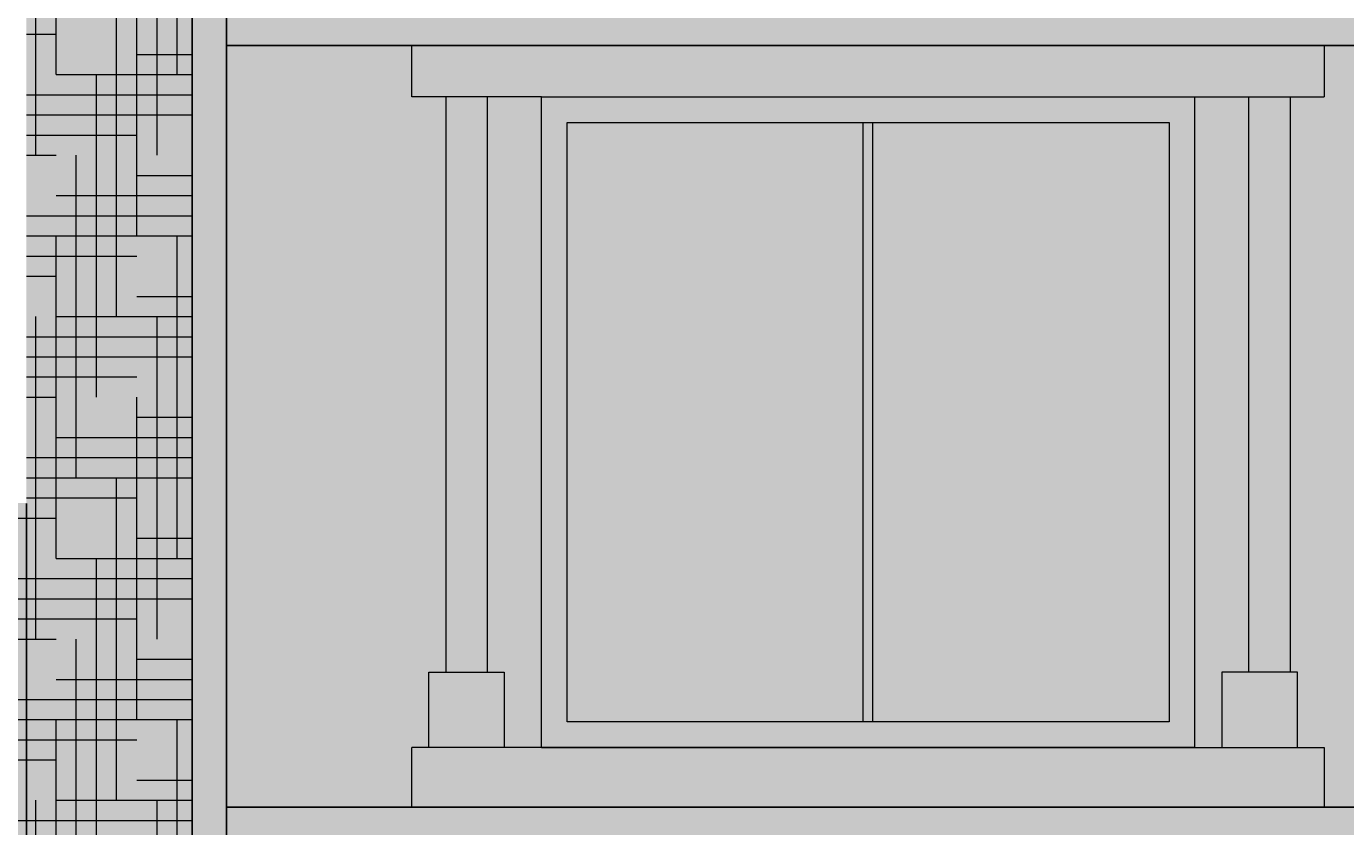
# Model space of a CAD drawing. Units: inches. Extents: x 3024 to 4744, y 1110 to 2100.
# Tile 15 of 29: x 3450 to 3657, y 1279 to 1405. Entities that reach past the tile are written whole.
import ezdxf

# ---------------------------------------------------------------- set-up
doc = ezdxf.new("R2010")
doc.units = ezdxf.units.IN
for name, color, linetype, lineweight in [('A-ANNO-DIMS', 2, 'Continuous', 18), ('A-ELEV', 7, 'Continuous', 25), ('A-ELEV-PATT', 252, 'Continuous', 13), ('A-GLAZ', 4, 'Continuous', 18)]:
    doc.layers.add(name, color=color, linetype=linetype, lineweight=lineweight)
doc.styles.get("Standard").update_dxf_attribs({"font": 'arial.ttf'})
doc.dimstyles.get("Standard").update_dxf_attribs({"dimtxt": 0.18, "dimasz": 0.18, "dimexe": 0.18, "dimexo": 0.0625, "dimgap": 0.09, "dimtad": 0, "dimtih": 1, "dimtoh": 1, "dimdec": 1, "dimzin": 0, "dimdsep": 46, "dimlunit": 3, "dimtxsty": 'Standard', "dimcen": 0.09, "dimadec": 0, "dimazin": 0, "dimtfac": 1, "dimtdec": 1, "dimtofl": 0, "dimtmove": 0, "dimatfit": 3, "dimfxl": 1, "dimtolj": 1, "dimtzin": 0, "dimarcsym": 0})

# ---------------------------------------------------------------- blocks, each defined once
blk = doc.blocks.new('WIN-BALCONY-A')
for p, q in [((3169.4, 1897.49), (3148.97, 1897.49)), ((3169.4, 1897.49), (3148.97, 1897.49)), ((3169.4, 1897.49), (3292.61, 1897.49)), ((3169.4, 1897.49), (3292.61, 1897.49)), ((3169.4, 1795.04), (3148.97, 1795.04)), ((3169.4, 1795.04), (3148.97, 1795.04)), ((3169.4, 1795.04), (3292.61, 1795.04)), ((3169.4, 1795.04), (3292.61, 1795.04))]:
    blk.add_line(p, q)
for points in [[(3148.97, 1897.49), (3148.97, 1905.61), (3292.61, 1905.61), (3292.61, 1897.49)], [(3148.97, 1897.49), (3148.97, 1905.61), (3292.61, 1905.61), (3292.61, 1897.49)], [(3292.61, 1795.04), (3292.61, 1785.61), (3148.97, 1785.61), (3148.97, 1795.04)], [(3292.61, 1795.04), (3292.61, 1785.61), (3148.97, 1785.61), (3148.97, 1795.04)]]:
    blk.add_lwpolyline(points)
for points in [[(3154.33, 1806.87), (3160.86, 1806.87), (3160.86, 1897.49), (3154.33, 1897.49)], [(3154.33, 1806.87), (3160.86, 1806.87), (3160.86, 1897.49), (3154.33, 1897.49)], [(3272.18, 1795.04), (3169.4, 1795.04), (3169.4, 1897.49), (3272.18, 1897.49)], [(3272.18, 1795.04), (3169.4, 1795.04), (3169.4, 1897.49), (3272.18, 1897.49)], [(3287.25, 1806.87), (3280.72, 1806.87), (3280.72, 1897.49), (3287.25, 1897.49)], [(3287.25, 1806.87), (3280.72, 1806.87), (3280.72, 1897.49), (3287.25, 1897.49)], [(3268.18, 1799.04), (3173.4, 1799.04), (3173.4, 1893.49), (3268.18, 1893.49)], [(3268.18, 1799.04), (3173.4, 1799.04), (3173.4, 1893.49), (3268.18, 1893.49)], [(3220.05, 1893.49), (3221.52, 1893.49), (3221.52, 1799.04), (3220.05, 1799.04)], [(3220.05, 1893.49), (3221.52, 1893.49), (3221.52, 1799.04), (3220.05, 1799.04)], [(3163.53, 1795.04), (3151.66, 1795.04), (3151.66, 1806.87), (3163.53, 1806.87)], [(3163.53, 1795.04), (3151.66, 1795.04), (3151.66, 1806.87), (3163.53, 1806.87)], [(3276.51, 1795.04), (3288.38, 1795.04), (3288.38, 1806.87), (3276.51, 1806.87)], [(3276.51, 1795.04), (3288.38, 1795.04), (3288.38, 1806.87), (3276.51, 1806.87)]]:
    blk.add_lwpolyline(points, close=True)
blk = doc.blocks.new('*D57')
at = {"layer": 'A-ANNO-DIMS', "color": 0, "lineweight": -2, "transparency": 16777216}
for p, q in [((3361.22, 1329.46), (3361.22, 1109.93)), ((3449.72, 1329.46), (3449.72, 1109.93)), ((3361.4, 1110.11), (3405.15, 1110.11)), ((3449.54, 1110.11), (3405.8, 1110.11))]:
    blk.add_line(p, q, dxfattribs=at)
at = {"layer": 'A-ANNO-DIMS', "color": 0, "transparency": 16777216}
for points in [[(3361.4, 1110.14), (3361.4, 1110.08), (3361.22, 1110.11)], [(3449.54, 1110.14), (3449.54, 1110.08), (3449.72, 1110.11)]]:
    blk.add_solid(points, dxfattribs=at)
at = {"layer": 'Defpoints', "color": 0, "transparency": 16777216}
for p in [(3361.22, 1329.52), (3449.72, 1329.52), (3449.72, 1110.11)]:
    blk.add_point(p, dxfattribs=at)
at = {"layer": 'A-ANNO-DIMS', "color": 0, "transparency": 16777216, "insert": (3405.47, 1110.11), "char_height": 0.18, "attachment_point": 5}
blk.add_mtext('\\A1;88.5', dxfattribs=at)
blk = doc.blocks.new('*D58')
at = {"layer": 'A-ANNO-DIMS', "color": 0, "lineweight": -2, "transparency": 16777216}
for p, q in [((3449.72, 1329.46), (3449.72, 1109.93)), ((3481.24, 1155.55), (3481.24, 1109.93)), ((3449.9, 1110.11), (3465.09, 1110.11)), ((3481.06, 1110.11), (3465.87, 1110.11))]:
    blk.add_line(p, q, dxfattribs=at)
at = {"layer": 'A-ANNO-DIMS', "color": 0, "transparency": 16777216}
for points in [[(3449.9, 1110.14), (3449.9, 1110.08), (3449.72, 1110.11)], [(3481.06, 1110.14), (3481.06, 1110.08), (3481.24, 1110.11)]]:
    blk.add_solid(points, dxfattribs=at)
at = {"layer": 'Defpoints', "color": 0, "transparency": 16777216}
for p in [(3449.72, 1329.52), (3481.24, 1155.61), (3481.24, 1110.11)]:
    blk.add_point(p, dxfattribs=at)
at = {"layer": 'A-ANNO-DIMS', "color": 0, "transparency": 16777216, "insert": (3465.48, 1110.11), "char_height": 0.18, "attachment_point": 5}
blk.add_mtext('\\A1;31.52', dxfattribs=at)
blk = doc.blocks.new('*D64')
at = {"layer": 'A-ANNO-DIMS', "color": 0, "lineweight": -2, "transparency": 16777216}
for p, q in [((3069.79, 1241.5), (3069.79, 2100.44)), ((3069.97, 2100.26), (3405.08, 2100.26)), ((3740.97, 2100.26), (3405.87, 2100.26)), ((3741.15, 1241.5), (3741.15, 2100.44))]:
    blk.add_line(p, q, dxfattribs=at)
at = {"layer": 'A-ANNO-DIMS', "color": 0, "transparency": 16777216}
for points in [[(3069.97, 2100.29), (3069.97, 2100.23), (3069.79, 2100.26)], [(3740.97, 2100.29), (3740.97, 2100.23), (3741.15, 2100.26)]]:
    blk.add_solid(points, dxfattribs=at)
at = {"layer": 'Defpoints', "color": 0, "transparency": 16777216}
for p in [(3741.15, 2100.26), (3069.79, 1241.43), (3741.15, 1241.43)]:
    blk.add_point(p, dxfattribs=at)
at = {"layer": 'A-ANNO-DIMS', "color": 0, "transparency": 16777216, "insert": (3405.47, 2100.26), "char_height": 0.18, "attachment_point": 5}
blk.add_mtext('\\A1;671.4', dxfattribs=at)
blk = doc.blocks.new('*D75')
at = {"layer": 'A-ANNO-DIMS', "color": 0, "lineweight": -2, "transparency": 16777216}
for p, q in [((3491.89, 2054.76), (3786.83, 2054.76)), ((3786.65, 2054.58), (3786.65, 1605.37)), ((3786.65, 1155.79), (3786.65, 1605)), ((3741.21, 1155.61), (3786.83, 1155.61))]:
    blk.add_line(p, q, dxfattribs=at)
at = {"layer": 'A-ANNO-DIMS', "color": 0, "transparency": 16777216}
for points in [[(3786.62, 2054.58), (3786.68, 2054.58), (3786.65, 2054.76)], [(3786.62, 1155.79), (3786.68, 1155.79), (3786.65, 1155.61)]]:
    blk.add_solid(points, dxfattribs=at)
at = {"layer": 'Defpoints', "color": 0, "transparency": 16777216}
for p in [(3491.83, 2054.76), (3786.65, 2054.76), (3741.15, 1155.61)]:
    blk.add_point(p, dxfattribs=at)
at = {"layer": 'A-ANNO-DIMS', "color": 0, "transparency": 16777216, "insert": (3786.65, 1605.18), "char_height": 0.18, "attachment_point": 5}
blk.add_mtext('\\A1;899.1', dxfattribs=at)

msp = doc.modelspace()

# ---------------------------------------------------------------- hatches: boundary and pattern name
at = {"layer": 'A-ELEV-PATT'}
h = msp.add_hatch(color=256, dxfattribs=at)
h.dxf.hatch_style = 1
h.paths.add_polyline_path([(3491.8271, 2054.7584), (3320.5658, 2054.7584), (3320.5658, 2043.5286), (3491.8271, 2043.5286)])
h.paths.add_polyline_path([(3292.6051, 1905.6112), (3148.9694, 1905.6112), (3148.9694, 1897.4879), (3169.3964, 1897.4879), (3292.6051, 1897.4879)])
h.paths.add_polyline_path([(3292.6051, 1795.0431), (3169.3964, 1795.0431), (3148.9694, 1795.0431), (3148.9694, 1785.6112), (3292.6051, 1785.6112)])
h.paths.add_polyline_path([(3292.6051, 1779.6112), (3148.9694, 1779.6112), (3148.9694, 1771.4879), (3169.3964, 1771.4879), (3292.6051, 1771.4879)])
h.paths.add_polyline_path([(3292.6051, 1669.0431), (3169.3964, 1669.0431), (3148.9694, 1669.0431), (3148.9694, 1659.6112), (3292.6051, 1659.6112)])
h.paths.add_polyline_path([(3292.6051, 1653.6112), (3148.9694, 1653.6112), (3148.9694, 1645.4879), (3169.3964, 1645.4879), (3292.6051, 1645.4879)])
h.paths.add_polyline_path([(3292.6051, 1543.0431), (3169.3964, 1543.0431), (3148.9694, 1543.0431), (3148.9694, 1533.6112), (3292.6051, 1533.6112)])
h.paths.add_polyline_path([(3292.6051, 1527.6112), (3148.9694, 1527.6112), (3148.9694, 1519.4879), (3169.3964, 1519.4879), (3292.6051, 1519.4879)])
h.paths.add_polyline_path([(3292.6051, 1401.6112), (3148.9694, 1401.6112), (3148.9694, 1393.4879), (3169.3964, 1393.4879), (3292.6051, 1393.4879)])
h.paths.add_polyline_path([(3292.6051, 1417.0431), (3169.3964, 1417.0431), (3148.9694, 1417.0431), (3148.9694, 1407.6112), (3292.6051, 1407.6112)])
h.paths.add_polyline_path([(3292.6051, 1291.0431), (3169.3964, 1291.0431), (3148.9694, 1291.0431), (3148.9694, 1281.6112), (3292.6051, 1281.6112)])
h.paths.add_polyline_path([(3654.037, 1165.0431), (3530.8283, 1165.0431), (3510.4013, 1165.0431), (3510.4013, 1155.6112), (3654.037, 1155.6112)])
h.paths.add_polyline_path([(3654.037, 1275.6112), (3510.4013, 1275.6112), (3510.4013, 1267.4879), (3530.8283, 1267.4879), (3654.037, 1267.4879)])
h.paths.add_polyline_path([(3654.037, 1291.0431), (3530.8283, 1291.0431), (3510.4013, 1291.0431), (3510.4013, 1281.6112), (3654.037, 1281.6112)])
h.paths.add_polyline_path([(3654.037, 1417.0431), (3530.8283, 1417.0431), (3510.4013, 1417.0431), (3510.4013, 1407.6112), (3654.037, 1407.6112)])
h.paths.add_polyline_path([(3654.037, 1401.6112), (3510.4013, 1401.6112), (3510.4013, 1393.4879), (3530.8283, 1393.4879), (3654.037, 1393.4879)])
h.paths.add_polyline_path([(3654.037, 1543.0431), (3530.8283, 1543.0431), (3510.4013, 1543.0431), (3510.4013, 1533.6112), (3654.037, 1533.6112)])
h.paths.add_polyline_path([(3654.037, 1527.6112), (3510.4013, 1527.6112), (3510.4013, 1519.4879), (3530.8283, 1519.4879), (3654.037, 1519.4879)])
h.paths.add_polyline_path([(3654.037, 1653.6112), (3510.4013, 1653.6112), (3510.4013, 1645.4879), (3530.8283, 1645.4879), (3654.037, 1645.4879)])
h.paths.add_polyline_path([(3654.037, 1669.0431), (3530.8283, 1669.0431), (3510.4013, 1669.0431), (3510.4013, 1659.6112), (3654.037, 1659.6112)])
h.paths.add_polyline_path([(3654.037, 1779.6112), (3510.4013, 1779.6112), (3510.4013, 1771.4879), (3530.8283, 1771.4879), (3654.037, 1771.4879)])
h.paths.add_polyline_path([(3654.037, 1795.0431), (3530.8283, 1795.0431), (3510.4013, 1795.0431), (3510.4013, 1785.6112), (3654.037, 1785.6112)])
h.paths.add_polyline_path([(3654.037, 1905.6112), (3510.4013, 1905.6112), (3510.4013, 1897.4879), (3530.8283, 1897.4879), (3654.037, 1897.4879)])
h = msp.add_hatch(color=256, dxfattribs=at)
h.dxf.hatch_style = 1
h.paths.add_polyline_path([(3335.1044, 2043.5286), (3329.7033, 2043.5286), (3329.7033, 1155.6112), (3335.1044, 1155.6112)])
h.paths.add_polyline_path([(3481.2411, 2043.5286), (3335.1044, 2043.5286), (3335.1044, 1155.6112), (3481.2411, 1155.6112)])
h.paths.add_polyline_path([(3449.7202, 1329.5246), (3361.2242, 1329.5246), (3361.2242, 1436.6064), (3449.7202, 1436.6064)], flags=16)
h.paths.add_polyline_path([(3445.7202, 1333.5246), (3365.2242, 1333.5246), (3365.2242, 1432.6064), (3445.7202, 1432.6064)], flags=0)
h.paths.add_polyline_path([(3449.7202, 1455.5246), (3361.2242, 1455.5246), (3361.2242, 1562.6064), (3449.7202, 1562.6064)], flags=16)
h.paths.add_polyline_path([(3445.7202, 1459.5246), (3365.2242, 1459.5246), (3365.2242, 1558.6064), (3445.7202, 1558.6064)], flags=0)
h.paths.add_polyline_path([(3449.7202, 1581.5246), (3361.2242, 1581.5246), (3361.2242, 1688.6064), (3449.7202, 1688.6064)], flags=16)
h.paths.add_polyline_path([(3445.7202, 1585.5246), (3365.2242, 1585.5246), (3365.2242, 1684.6064), (3445.7202, 1684.6064)], flags=0)
h.paths.add_polyline_path([(3449.7202, 1707.5246), (3361.2242, 1707.5246), (3361.2242, 1814.6064), (3449.7202, 1814.6064)], flags=16)
h.paths.add_polyline_path([(3445.7202, 1711.5246), (3365.2242, 1711.5246), (3365.2242, 1810.6064), (3445.7202, 1810.6064)], flags=0)
h.paths.add_polyline_path([(3449.7202, 1833.5246), (3361.2242, 1833.5246), (3361.2242, 1940.6064), (3449.7202, 1940.6064)], flags=16)
h.paths.add_polyline_path([(3445.7202, 1837.5246), (3365.2242, 1837.5246), (3365.2242, 1936.6064), (3445.7202, 1936.6064)], flags=0)
h = msp.add_hatch(color=256, dxfattribs=at)
h.dxf.hatch_style = 1
h.paths.add_polyline_path([(3475.84, 2043.5286), (3335.1044, 2043.5286), (3335.1044, 1155.6112), (3475.84, 1155.6112)])
h.paths.add_polyline_path([(3449.7202, 1940.6064), (3449.7202, 1833.5246), (3361.2242, 1833.5246), (3361.2242, 1940.6064)], flags=16)
h.paths.add_polyline_path([(3445.7202, 1936.6064), (3445.7202, 1837.5246), (3365.2242, 1837.5246), (3365.2242, 1936.6064)], flags=0)
h.paths.add_polyline_path([(3449.7202, 1814.6064), (3449.7202, 1707.5246), (3361.2242, 1707.5246), (3361.2242, 1814.6064)], flags=16)
h.paths.add_polyline_path([(3445.7202, 1810.6064), (3445.7202, 1711.5246), (3365.2242, 1711.5246), (3365.2242, 1810.6064)], flags=0)
h.paths.add_polyline_path([(3449.7202, 1688.6064), (3449.7202, 1581.5246), (3361.2242, 1581.5246), (3361.2242, 1688.6064)], flags=16)
h.paths.add_polyline_path([(3445.7202, 1684.6064), (3445.7202, 1585.5246), (3365.2242, 1585.5246), (3365.2242, 1684.6064)], flags=0)
h.paths.add_polyline_path([(3449.7202, 1562.6064), (3449.7202, 1455.5246), (3361.2242, 1455.5246), (3361.2242, 1562.6064)], flags=16)
h.paths.add_polyline_path([(3445.7202, 1558.6064), (3445.7202, 1459.5246), (3365.2242, 1459.5246), (3365.2242, 1558.6064)], flags=0)
h.paths.add_polyline_path([(3449.7202, 1436.6064), (3449.7202, 1329.5246), (3361.2242, 1329.5246), (3361.2242, 1436.6064)], flags=16)
h.paths.add_polyline_path([(3445.7202, 1432.6064), (3445.7202, 1333.5246), (3365.2242, 1333.5246), (3365.2242, 1432.6064)], flags=0)
h = msp.add_hatch(dxfattribs=at)
h.set_pattern_fill('HOUND', color=256, scale=2)
h.paths.add_polyline_path([(3475.84, 2043.5286), (3335.1044, 2043.5286), (3335.1044, 1155.6112), (3475.84, 1155.6112)])
h.paths.add_polyline_path([(3449.7202, 1940.6064), (3449.7202, 1833.5246), (3361.2242, 1833.5246), (3361.2242, 1940.6064)], flags=16)
h.paths.add_polyline_path([(3445.7202, 1936.6064), (3445.7202, 1837.5246), (3365.2242, 1837.5246), (3365.2242, 1936.6064)], flags=0)
h.paths.add_polyline_path([(3449.7202, 1814.6064), (3449.7202, 1707.5246), (3361.2242, 1707.5246), (3361.2242, 1814.6064)], flags=16)
h.paths.add_polyline_path([(3445.7202, 1810.6064), (3445.7202, 1711.5246), (3365.2242, 1711.5246), (3365.2242, 1810.6064)], flags=0)
h.paths.add_polyline_path([(3449.7202, 1688.6064), (3449.7202, 1581.5246), (3361.2242, 1581.5246), (3361.2242, 1688.6064)], flags=16)
h.paths.add_polyline_path([(3445.7202, 1684.6064), (3445.7202, 1585.5246), (3365.2242, 1585.5246), (3365.2242, 1684.6064)], flags=0)
h.paths.add_polyline_path([(3449.7202, 1562.6064), (3449.7202, 1455.5246), (3361.2242, 1455.5246), (3361.2242, 1562.6064)], flags=16)
h.paths.add_polyline_path([(3445.7202, 1558.6064), (3445.7202, 1459.5246), (3365.2242, 1459.5246), (3365.2242, 1558.6064)], flags=0)
h.paths.add_polyline_path([(3449.7202, 1436.6064), (3449.7202, 1329.5246), (3361.2242, 1329.5246), (3361.2242, 1436.6064)], flags=16)
h.paths.add_polyline_path([(3445.7202, 1432.6064), (3445.7202, 1333.5246), (3365.2242, 1333.5246), (3365.2242, 1432.6064)], flags=0)
h = msp.add_hatch(color=256, dxfattribs=at)
h.dxf.hatch_style = 1
h.paths.add_polyline_path([(3154.3287, 1897.4879), (3148.9694, 1897.4879), (3148.9694, 1905.6112), (3105.4722, 1905.6112), (3105.4722, 1785.6112), (3148.9694, 1785.6112), (3148.9694, 1795.0431), (3151.6604, 1795.0431), (3151.6604, 1806.8674), (3154.3287, 1806.8674)])
h.paths.add_polyline_path([(3329.7033, 1905.6112), (3292.6051, 1905.6112), (3292.6051, 1897.4879), (3287.2458, 1897.4879), (3287.2458, 1806.8674), (3288.3759, 1806.8674), (3288.3759, 1795.0431), (3292.6051, 1795.0431), (3292.6051, 1785.6112), (3329.7033, 1785.6112)])
h.paths.add_polyline_path([(3154.3287, 1771.4879), (3148.9694, 1771.4879), (3148.9694, 1779.6112), (3105.4722, 1779.6112), (3105.4722, 1659.6112), (3148.9694, 1659.6112), (3148.9694, 1669.0431), (3151.6604, 1669.0431), (3151.6604, 1680.8674), (3154.3287, 1680.8674)])
h.paths.add_polyline_path([(3329.7033, 1779.6112), (3292.6051, 1779.6112), (3292.6051, 1771.4879), (3287.2458, 1771.4879), (3287.2458, 1680.8674), (3288.3759, 1680.8674), (3288.3759, 1669.0431), (3292.6051, 1669.0431), (3292.6051, 1659.6112), (3329.7033, 1659.6112)])
h.paths.add_polyline_path([(3154.3287, 1645.4879), (3148.9694, 1645.4879), (3148.9694, 1653.6112), (3105.4722, 1653.6112), (3105.4722, 1533.6112), (3148.9694, 1533.6112), (3148.9694, 1543.0431), (3151.6604, 1543.0431), (3151.6604, 1554.8674), (3154.3287, 1554.8674)])
h.paths.add_polyline_path([(3329.7033, 1653.6112), (3292.6051, 1653.6112), (3292.6051, 1645.4879), (3287.2458, 1645.4879), (3287.2458, 1554.8674), (3288.3759, 1554.8674), (3288.3759, 1543.0431), (3292.6051, 1543.0431), (3292.6051, 1533.6112), (3329.7033, 1533.6112)])
h.paths.add_polyline_path([(3329.7033, 1527.6112), (3292.6051, 1527.6112), (3292.6051, 1519.4879), (3287.2458, 1519.4879), (3287.2458, 1428.8674), (3288.3759, 1428.8674), (3288.3759, 1417.0431), (3292.6051, 1417.0431), (3292.6051, 1407.6112), (3329.7033, 1407.6112)])
h.paths.add_polyline_path([(3329.7033, 1401.6112), (3292.6051, 1401.6112), (3292.6051, 1393.4879), (3287.2458, 1393.4879), (3287.2458, 1302.8674), (3288.3759, 1302.8674), (3288.3759, 1291.0431), (3292.6051, 1291.0431), (3292.6051, 1281.6112), (3329.7033, 1281.6112)])
h.paths.add_polyline_path([(3154.3287, 1393.4879), (3148.9694, 1393.4879), (3148.9694, 1401.6112), (3105.4722, 1401.6112), (3105.4722, 1281.6112), (3148.9694, 1281.6112), (3148.9694, 1291.0431), (3151.6604, 1291.0431), (3151.6604, 1302.8674), (3154.3287, 1302.8674)])
h.paths.add_polyline_path([(3154.3287, 1519.4879), (3148.9694, 1519.4879), (3148.9694, 1527.6112), (3105.4722, 1527.6112), (3105.4722, 1407.6112), (3148.9694, 1407.6112), (3148.9694, 1417.0431), (3151.6604, 1417.0431), (3151.6604, 1428.8674), (3154.3287, 1428.8674)])
h.paths.add_polyline_path([(3515.7606, 1897.4879), (3510.4013, 1897.4879), (3510.4013, 1905.6112), (3481.2411, 1905.6112), (3481.2411, 1785.6112), (3510.4013, 1785.6112), (3510.4013, 1795.0431), (3513.0923, 1795.0431), (3513.0923, 1806.8674), (3515.7606, 1806.8674)])
h.paths.add_polyline_path([(3688.5588, 1905.6112), (3654.037, 1905.6112), (3654.037, 1897.4879), (3648.6777, 1897.4879), (3648.6777, 1806.8674), (3649.8078, 1806.8674), (3649.8078, 1795.0431), (3654.037, 1795.0431), (3654.037, 1785.6112), (3688.5588, 1785.6112)])
h.paths.add_polyline_path([(3515.7606, 1771.4879), (3510.4013, 1771.4879), (3510.4013, 1779.6112), (3481.2411, 1779.6112), (3481.2411, 1659.6112), (3510.4013, 1659.6112), (3510.4013, 1669.0431), (3513.0923, 1669.0431), (3513.0923, 1680.8674), (3515.7606, 1680.8674)])
h.paths.add_polyline_path([(3688.5588, 1779.6112), (3654.037, 1779.6112), (3654.037, 1771.4879), (3648.6777, 1771.4879), (3648.6777, 1680.8674), (3649.8078, 1680.8674), (3649.8078, 1669.0431), (3654.037, 1669.0431), (3654.037, 1659.6112), (3688.5588, 1659.6112)])
h.paths.add_polyline_path([(3515.7606, 1645.4879), (3510.4013, 1645.4879), (3510.4013, 1653.6112), (3481.2411, 1653.6112), (3481.2411, 1533.6112), (3510.4013, 1533.6112), (3510.4013, 1543.0431), (3513.0923, 1543.0431), (3513.0923, 1554.8674), (3515.7606, 1554.8674)])
h.paths.add_polyline_path([(3688.5588, 1653.6112), (3654.037, 1653.6112), (3654.037, 1645.4879), (3648.6777, 1645.4879), (3648.6777, 1554.8674), (3649.8078, 1554.8674), (3649.8078, 1543.0431), (3654.037, 1543.0431), (3654.037, 1533.6112), (3688.5588, 1533.6112)])
h.paths.add_polyline_path([(3515.7606, 1519.4879), (3510.4013, 1519.4879), (3510.4013, 1527.6112), (3481.2411, 1527.6112), (3481.2411, 1407.6112), (3510.4013, 1407.6112), (3510.4013, 1417.0431), (3513.0923, 1417.0431), (3513.0923, 1428.8674), (3515.7606, 1428.8674)])
h.paths.add_polyline_path([(3688.5588, 1527.6112), (3654.037, 1527.6112), (3654.037, 1519.4879), (3648.6777, 1519.4879), (3648.6777, 1428.8674), (3649.8078, 1428.8674), (3649.8078, 1417.0431), (3654.037, 1417.0431), (3654.037, 1407.6112), (3688.5588, 1407.6112)])
h.paths.add_polyline_path([(3515.7606, 1393.4879), (3510.4013, 1393.4879), (3510.4013, 1401.6112), (3481.2411, 1401.6112), (3481.2411, 1281.6112), (3510.4013, 1281.6112), (3510.4013, 1291.0431), (3513.0923, 1291.0431), (3513.0923, 1302.8674), (3515.7606, 1302.8674)])
h.paths.add_polyline_path([(3688.5588, 1401.6112), (3654.037, 1401.6112), (3654.037, 1393.4879), (3648.6777, 1393.4879), (3648.6777, 1302.8674), (3649.8078, 1302.8674), (3649.8078, 1291.0431), (3654.037, 1291.0431), (3654.037, 1281.6112), (3688.5588, 1281.6112)])
h.paths.add_polyline_path([(3515.7606, 1267.4879), (3510.4013, 1267.4879), (3510.4013, 1275.6112), (3481.2411, 1275.6112), (3481.2411, 1155.6112), (3510.4013, 1155.6112), (3510.4013, 1165.0431), (3513.0923, 1165.0431), (3513.0923, 1176.8674), (3515.7606, 1176.8674)])
h.paths.add_polyline_path([(3688.5588, 1275.6112), (3654.037, 1275.6112), (3654.037, 1267.4879), (3648.6777, 1267.4879), (3648.6777, 1176.8674), (3649.8078, 1176.8674), (3649.8078, 1165.0431), (3654.037, 1165.0431), (3654.037, 1155.6112), (3688.5588, 1155.6112)])
h.paths.add_polyline_path([(3112.3838, 1275.6112), (3105.4722, 1275.6112), (3105.4722, 1171.0239), (3112.3838, 1171.0239)])
h = msp.add_hatch(color=256, dxfattribs=at)
h.dxf.hatch_style = 1
h.paths.add_polyline_path([(3160.8586, 1897.4879), (3154.3287, 1897.4879), (3154.3287, 1806.8674), (3160.8586, 1806.8674)])
h.paths.add_polyline_path([(3287.2458, 1897.4879), (3280.716, 1897.4879), (3280.716, 1806.8674), (3287.2458, 1806.8674)])
h.paths.add_polyline_path([(3160.8586, 1771.4879), (3154.3287, 1771.4879), (3154.3287, 1680.8674), (3160.8586, 1680.8674)])
h.paths.add_polyline_path([(3287.2458, 1771.4879), (3280.716, 1771.4879), (3280.716, 1680.8674), (3287.2458, 1680.8674)])
h.paths.add_polyline_path([(3160.8586, 1645.4879), (3154.3287, 1645.4879), (3154.3287, 1554.8674), (3160.8586, 1554.8674)])
h.paths.add_polyline_path([(3287.2458, 1645.4879), (3280.716, 1645.4879), (3280.716, 1554.8674), (3287.2458, 1554.8674)])
h.paths.add_polyline_path([(3160.8586, 1519.4879), (3154.3287, 1519.4879), (3154.3287, 1428.8674), (3160.8586, 1428.8674)])
h.paths.add_polyline_path([(3287.2458, 1519.4879), (3280.716, 1519.4879), (3280.716, 1428.8674), (3287.2458, 1428.8674)])
h.paths.add_polyline_path([(3160.8586, 1393.4879), (3154.3287, 1393.4879), (3154.3287, 1302.8674), (3160.8586, 1302.8674)])
h.paths.add_polyline_path([(3287.2458, 1393.4879), (3280.716, 1393.4879), (3280.716, 1302.8674), (3287.2458, 1302.8674)])
h.paths.add_polyline_path([(3648.6777, 1267.4879), (3642.1479, 1267.4879), (3642.1479, 1176.8674), (3648.6777, 1176.8674)])
h.paths.add_polyline_path([(3522.2905, 1267.4879), (3515.7606, 1267.4879), (3515.7606, 1176.8674), (3522.2905, 1176.8674)])
h.paths.add_polyline_path([(3522.2905, 1393.4879), (3515.7606, 1393.4879), (3515.7606, 1302.8674), (3522.2905, 1302.8674)])
h.paths.add_polyline_path([(3648.6777, 1393.4879), (3642.1479, 1393.4879), (3642.1479, 1302.8674), (3648.6777, 1302.8674)])
h.paths.add_polyline_path([(3522.2905, 1519.4879), (3515.7606, 1519.4879), (3515.7606, 1428.8674), (3522.2905, 1428.8674)])
h.paths.add_polyline_path([(3648.6777, 1519.4879), (3642.1479, 1519.4879), (3642.1479, 1428.8674), (3648.6777, 1428.8674)])
h.paths.add_polyline_path([(3522.2905, 1645.4879), (3515.7606, 1645.4879), (3515.7606, 1554.8674), (3522.2905, 1554.8674)])
h.paths.add_polyline_path([(3522.2905, 1771.4879), (3515.7606, 1771.4879), (3515.7606, 1680.8674), (3522.2905, 1680.8674)])
h.paths.add_polyline_path([(3648.6777, 1645.4879), (3642.1479, 1645.4879), (3642.1479, 1554.8674), (3648.6777, 1554.8674)])
h.paths.add_polyline_path([(3648.6777, 1771.4879), (3642.1479, 1771.4879), (3642.1479, 1680.8674), (3648.6777, 1680.8674)])
h.paths.add_polyline_path([(3648.6777, 1897.4879), (3642.1479, 1897.4879), (3642.1479, 1806.8674), (3648.6777, 1806.8674)])
h.paths.add_polyline_path([(3522.2905, 1897.4879), (3515.7606, 1897.4879), (3515.7606, 1806.8674), (3522.2905, 1806.8674)])
h = msp.add_hatch(color=256, dxfattribs=at)
h.dxf.hatch_style = 1
h.paths.add_polyline_path([(3169.3964, 1897.4879), (3160.8586, 1897.4879), (3160.8586, 1806.8674), (3163.5269, 1806.8674), (3163.5269, 1795.0431), (3169.3964, 1795.0431)])
h.paths.add_polyline_path([(3280.716, 1897.4879), (3272.1781, 1897.4879), (3272.1781, 1795.0431), (3276.5094, 1795.0431), (3276.5094, 1806.8674), (3280.716, 1806.8674)])
h.paths.add_polyline_path([(3280.716, 1771.4879), (3272.1781, 1771.4879), (3272.1781, 1669.0431), (3276.5094, 1669.0431), (3276.5094, 1680.8674), (3280.716, 1680.8674)])
h.paths.add_polyline_path([(3169.3964, 1771.4879), (3160.8586, 1771.4879), (3160.8586, 1680.8674), (3163.5269, 1680.8674), (3163.5269, 1669.0431), (3169.3964, 1669.0431)])
h.paths.add_polyline_path([(3169.3964, 1645.4879), (3160.8586, 1645.4879), (3160.8586, 1554.8674), (3163.5269, 1554.8674), (3163.5269, 1543.0431), (3169.3964, 1543.0431)])
h.paths.add_polyline_path([(3280.716, 1645.4879), (3272.1781, 1645.4879), (3272.1781, 1543.0431), (3276.5094, 1543.0431), (3276.5094, 1554.8674), (3280.716, 1554.8674)])
h.paths.add_polyline_path([(3169.3964, 1519.4879), (3160.8586, 1519.4879), (3160.8586, 1428.8674), (3163.5269, 1428.8674), (3163.5269, 1417.0431), (3169.3964, 1417.0431)])
h.paths.add_polyline_path([(3280.716, 1519.4879), (3272.1781, 1519.4879), (3272.1781, 1417.0431), (3276.5094, 1417.0431), (3276.5094, 1428.8674), (3280.716, 1428.8674)])
h.paths.add_polyline_path([(3169.3964, 1393.4879), (3160.8586, 1393.4879), (3160.8586, 1302.8674), (3163.5269, 1302.8674), (3163.5269, 1291.0431), (3169.3964, 1291.0431)])
h.paths.add_polyline_path([(3280.716, 1393.4879), (3272.1781, 1393.4879), (3272.1781, 1291.0431), (3276.5094, 1291.0431), (3276.5094, 1302.8674), (3280.716, 1302.8674)])
h.paths.add_polyline_path([(3642.1479, 1267.4879), (3633.61, 1267.4879), (3633.61, 1165.0431), (3637.9413, 1165.0431), (3637.9413, 1176.8674), (3642.1479, 1176.8674)])
h.paths.add_polyline_path([(3530.8283, 1267.4879), (3522.2905, 1267.4879), (3522.2905, 1176.8674), (3524.9588, 1176.8674), (3524.9588, 1165.0431), (3530.8283, 1165.0431)])
h.paths.add_polyline_path([(3642.1479, 1393.4879), (3633.61, 1393.4879), (3633.61, 1291.0431), (3637.9413, 1291.0431), (3637.9413, 1302.8674), (3642.1479, 1302.8674)])
h.paths.add_polyline_path([(3530.8283, 1393.4879), (3522.2905, 1393.4879), (3522.2905, 1302.8674), (3524.9588, 1302.8674), (3524.9588, 1291.0431), (3530.8283, 1291.0431)])
h.paths.add_polyline_path([(3530.8283, 1519.4879), (3522.2905, 1519.4879), (3522.2905, 1428.8674), (3524.9588, 1428.8674), (3524.9588, 1417.0431), (3530.8283, 1417.0431)])
h.paths.add_polyline_path([(3642.1479, 1519.4879), (3633.61, 1519.4879), (3633.61, 1417.0431), (3637.9413, 1417.0431), (3637.9413, 1428.8674), (3642.1479, 1428.8674)])
h.paths.add_polyline_path([(3530.8283, 1645.4879), (3522.2905, 1645.4879), (3522.2905, 1554.8674), (3524.9588, 1554.8674), (3524.9588, 1543.0431), (3530.8283, 1543.0431)])
h.paths.add_polyline_path([(3642.1479, 1645.4879), (3633.61, 1645.4879), (3633.61, 1543.0431), (3637.9413, 1543.0431), (3637.9413, 1554.8674), (3642.1479, 1554.8674)])
h.paths.add_polyline_path([(3642.1479, 1771.4879), (3633.61, 1771.4879), (3633.61, 1669.0431), (3637.9413, 1669.0431), (3637.9413, 1680.8674), (3642.1479, 1680.8674)])
h.paths.add_polyline_path([(3530.8283, 1771.4879), (3522.2905, 1771.4879), (3522.2905, 1680.8674), (3524.9588, 1680.8674), (3524.9588, 1669.0431), (3530.8283, 1669.0431)])
h.paths.add_polyline_path([(3530.8283, 1897.4879), (3522.2905, 1897.4879), (3522.2905, 1806.8674), (3524.9588, 1806.8674), (3524.9588, 1795.0431), (3530.8283, 1795.0431)])
h.paths.add_polyline_path([(3642.1479, 1897.4879), (3633.61, 1897.4879), (3633.61, 1795.0431), (3637.9413, 1795.0431), (3637.9413, 1806.8674), (3642.1479, 1806.8674)])
h = msp.add_hatch(color=256, dxfattribs=at)
h.dxf.hatch_style = 1
h.paths.add_polyline_path([(3220.0505, 1893.4879), (3173.3964, 1893.4879), (3173.3964, 1799.0431), (3220.0505, 1799.0431)])
h.paths.add_polyline_path([(3268.1781, 1893.4879), (3221.5241, 1893.4879), (3221.5241, 1799.0431), (3268.1781, 1799.0431)])
h.paths.add_polyline_path([(3581.4824, 1893.4879), (3534.8283, 1893.4879), (3534.8283, 1799.0431), (3581.4824, 1799.0431)])
h.paths.add_polyline_path([(3629.61, 1893.4879), (3582.956, 1893.4879), (3582.956, 1799.0431), (3629.61, 1799.0431)])
h.paths.add_polyline_path([(3581.4824, 1767.4879), (3534.8283, 1767.4879), (3534.8283, 1673.0431), (3581.4824, 1673.0431)])
h.paths.add_polyline_path([(3629.61, 1767.4879), (3582.956, 1767.4879), (3582.956, 1673.0431), (3629.61, 1673.0431)])
h.paths.add_polyline_path([(3581.4824, 1641.4879), (3534.8283, 1641.4879), (3534.8283, 1547.0431), (3581.4824, 1547.0431)])
h.paths.add_polyline_path([(3629.61, 1641.4879), (3582.956, 1641.4879), (3582.956, 1547.0431), (3629.61, 1547.0431)])
h.paths.add_polyline_path([(3629.61, 1515.4879), (3582.956, 1515.4879), (3582.956, 1421.0431), (3629.61, 1421.0431)])
h.paths.add_polyline_path([(3581.4824, 1515.4879), (3534.8283, 1515.4879), (3534.8283, 1421.0431), (3581.4824, 1421.0431)])
h.paths.add_polyline_path([(3629.61, 1389.4879), (3582.956, 1389.4879), (3582.956, 1295.0431), (3629.61, 1295.0431)])
h.paths.add_polyline_path([(3581.4824, 1389.4879), (3534.8283, 1389.4879), (3534.8283, 1295.0431), (3581.4824, 1295.0431)])
h.paths.add_polyline_path([(3629.61, 1263.4879), (3582.956, 1263.4879), (3582.956, 1169.0431), (3629.61, 1169.0431)])
h.paths.add_polyline_path([(3581.4824, 1263.4879), (3534.8283, 1263.4879), (3534.8283, 1169.0431), (3581.4824, 1169.0431)])
h.paths.add_polyline_path([(3220.0505, 1389.4879), (3173.3964, 1389.4879), (3173.3964, 1295.0431), (3220.0505, 1295.0431)])
h.paths.add_polyline_path([(3268.1781, 1389.4879), (3221.5241, 1389.4879), (3221.5241, 1295.0431), (3268.1781, 1295.0431)])
h.paths.add_polyline_path([(3220.0505, 1515.4879), (3173.3964, 1515.4879), (3173.3964, 1421.0431), (3220.0505, 1421.0431)])
h.paths.add_polyline_path([(3268.1781, 1515.4879), (3221.5241, 1515.4879), (3221.5241, 1421.0431), (3268.1781, 1421.0431)])
h.paths.add_polyline_path([(3220.0505, 1767.4879), (3173.3964, 1767.4879), (3173.3964, 1673.0431), (3220.0505, 1673.0431)])
h.paths.add_polyline_path([(3268.1781, 1767.4879), (3221.5241, 1767.4879), (3221.5241, 1673.0431), (3268.1781, 1673.0431)])
h.paths.add_polyline_path([(3220.0505, 1641.4879), (3173.3964, 1641.4879), (3173.3964, 1547.0431), (3220.0505, 1547.0431)])
h.paths.add_polyline_path([(3268.1781, 1641.4879), (3221.5241, 1641.4879), (3221.5241, 1547.0431), (3268.1781, 1547.0431)])
h = msp.add_hatch(color=256, dxfattribs=at)
h.dxf.hatch_style = 1
h.paths.add_polyline_path([(3163.5269, 1302.8674), (3151.6604, 1302.8674), (3151.6604, 1291.0431), (3163.5269, 1291.0431)])
h.paths.add_polyline_path([(3288.3759, 1302.8674), (3276.5094, 1302.8674), (3276.5094, 1291.0431), (3288.3759, 1291.0431)])
h.paths.add_polyline_path([(3288.3759, 1428.8674), (3276.5094, 1428.8674), (3276.5094, 1417.0431), (3288.3759, 1417.0431)])
h.paths.add_polyline_path([(3163.5269, 1428.8674), (3151.6604, 1428.8674), (3151.6604, 1417.0431), (3163.5269, 1417.0431)])
h.paths.add_polyline_path([(3163.5269, 1554.8674), (3151.6604, 1554.8674), (3151.6604, 1543.0431), (3163.5269, 1543.0431)])
h.paths.add_polyline_path([(3288.3759, 1554.8674), (3276.5094, 1554.8674), (3276.5094, 1543.0431), (3288.3759, 1543.0431)])
h.paths.add_polyline_path([(3163.5269, 1680.8674), (3151.6604, 1680.8674), (3151.6604, 1669.0431), (3163.5269, 1669.0431)])
h.paths.add_polyline_path([(3288.3759, 1680.8674), (3276.5094, 1680.8674), (3276.5094, 1669.0431), (3288.3759, 1669.0431)])
h.paths.add_polyline_path([(3163.5269, 1806.8674), (3151.6604, 1806.8674), (3151.6604, 1795.0431), (3163.5269, 1795.0431)])
h.paths.add_polyline_path([(3288.3759, 1806.8674), (3276.5094, 1806.8674), (3276.5094, 1795.0431), (3288.3759, 1795.0431)])
h.paths.add_polyline_path([(3524.9588, 1806.8674), (3513.0923, 1806.8674), (3513.0923, 1795.0431), (3524.9588, 1795.0431)])
h.paths.add_polyline_path([(3649.8078, 1806.8674), (3637.9413, 1806.8674), (3637.9413, 1795.0431), (3649.8078, 1795.0431)])
h.paths.add_polyline_path([(3524.9588, 1680.8674), (3513.0923, 1680.8674), (3513.0923, 1669.0431), (3524.9588, 1669.0431)])
h.paths.add_polyline_path([(3649.8078, 1680.8674), (3637.9413, 1680.8674), (3637.9413, 1669.0431), (3649.8078, 1669.0431)])
h.paths.add_polyline_path([(3524.9588, 1554.8674), (3513.0923, 1554.8674), (3513.0923, 1543.0431), (3524.9588, 1543.0431)])
h.paths.add_polyline_path([(3649.8078, 1554.8674), (3637.9413, 1554.8674), (3637.9413, 1543.0431), (3649.8078, 1543.0431)])
h.paths.add_polyline_path([(3524.9588, 1428.8674), (3513.0923, 1428.8674), (3513.0923, 1417.0431), (3524.9588, 1417.0431)])
h.paths.add_polyline_path([(3649.8078, 1428.8674), (3637.9413, 1428.8674), (3637.9413, 1417.0431), (3649.8078, 1417.0431)])
h.paths.add_polyline_path([(3524.9588, 1302.8674), (3513.0923, 1302.8674), (3513.0923, 1291.0431), (3524.9588, 1291.0431)])
h.paths.add_polyline_path([(3649.8078, 1302.8674), (3637.9413, 1302.8674), (3637.9413, 1291.0431), (3649.8078, 1291.0431)])
h.paths.add_polyline_path([(3524.9588, 1176.8674), (3513.0923, 1176.8674), (3513.0923, 1165.0431), (3524.9588, 1165.0431)])
h.paths.add_polyline_path([(3649.8078, 1176.8674), (3637.9413, 1176.8674), (3637.9413, 1165.0431), (3649.8078, 1165.0431)])
h = msp.add_hatch(color=256, dxfattribs=at)
h.dxf.hatch_style = 1
h.paths.add_polyline_path([(3688.5588, 1785.6112), (3481.2411, 1785.6112), (3481.2411, 1779.6112), (3688.5588, 1779.6112)])
h.paths.add_polyline_path([(3688.5588, 1659.6112), (3481.2411, 1659.6112), (3481.2411, 1653.6112), (3688.5588, 1653.6112)])
h.paths.add_polyline_path([(3688.5588, 1533.6112), (3481.2411, 1533.6112), (3481.2411, 1527.6112), (3688.5588, 1527.6112)])
h.paths.add_polyline_path([(3688.5588, 1407.6112), (3481.2411, 1407.6112), (3481.2411, 1401.6112), (3688.5588, 1401.6112)])
h.paths.add_polyline_path([(3688.5588, 1281.6112), (3481.2411, 1281.6112), (3481.2411, 1275.6112), (3688.5588, 1275.6112)])
h = msp.add_hatch(color=256, dxfattribs=at)
h.dxf.hatch_style = 1
h.paths.add_polyline_path([(3582.956, 1515.4879), (3581.4824, 1515.4879), (3581.4824, 1421.0431), (3582.956, 1421.0431)], flags=0)
h.paths.add_polyline_path([(3582.956, 1515.4879), (3582.956, 1421.0431), (3581.4824, 1421.0431), (3581.4824, 1515.4879)], flags=0)
h.paths.add_polyline_path([(3582.956, 1389.4879), (3581.4824, 1389.4879), (3581.4824, 1295.0431), (3582.956, 1295.0431)])
h = msp.add_hatch(color=256, dxfattribs=at)
h.dxf.hatch_style = 1
h.paths.add_polyline_path([(3582.956, 1389.4879), (3581.4824, 1389.4879), (3581.4824, 1295.0431), (3582.956, 1295.0431)], flags=0)
h.paths.add_polyline_path([(3633.61, 1393.4879), (3530.8283, 1393.4879), (3530.8283, 1291.0431), (3633.61, 1291.0431)])
h.paths.add_polyline_path([(3629.61, 1389.4879), (3629.61, 1295.0431), (3534.8283, 1295.0431), (3534.8283, 1389.4879)], flags=16)
h.paths.add_polyline_path([(3582.956, 1389.4879), (3582.956, 1295.0431), (3581.4824, 1295.0431), (3581.4824, 1389.4879)], flags=0)
h = msp.add_hatch(color=256, dxfattribs=at)
h.dxf.hatch_style = 1
h.paths.add_polyline_path([(3582.956, 1389.4879), (3581.4824, 1389.4879), (3581.4824, 1295.0431), (3582.956, 1295.0431)], flags=0)
h.paths.add_polyline_path([(3582.956, 1389.4879), (3582.956, 1295.0431), (3581.4824, 1295.0431), (3581.4824, 1389.4879)], flags=0)
h.paths.add_polyline_path([(3582.956, 1263.4879), (3581.4824, 1263.4879), (3581.4824, 1169.0431), (3582.956, 1169.0431)])

# ---------------------------------------------------------------- linework, layer by layer
at = {"layer": 'A-ELEV'}
for p, q in [((3688.5588, 1401.6112), (3481.2411, 1401.6112)), ((3688.5588, 1401.6112), (3481.2411, 1401.6112)), ((3481.2411, 1281.6112), (3688.5588, 1281.6112)), ((3481.2411, 1281.6112), (3688.5588, 1281.6112))]:
    msp.add_line(p, q, dxfattribs=at)
for points in [[(3481.2411, 1155.6112), (3329.7033, 1155.6112), (3329.7033, 2043.5286), (3481.2411, 2043.5286)], [(3481.2411, 1155.6112), (3329.7033, 1155.6112), (3329.7033, 2043.5286), (3481.2411, 2043.5286)], [(3475.84, 2043.5286), (3481.2411, 2043.5286), (3481.2411, 1155.6112), (3475.84, 1155.6112)], [(3475.84, 2043.5286), (3481.2411, 2043.5286), (3481.2411, 1155.6112), (3475.84, 1155.6112)], [(3475.84, 2043.5286), (3481.2411, 2043.5286), (3481.2411, 1155.6112), (3475.84, 1155.6112)]]:
    msp.add_lwpolyline(points, close=True, dxfattribs=at)

# ---------------------------------------------------------------- block references
at = {"layer": 'A-GLAZ'}
msp.add_blockref('WIN-BALCONY-A', (361.4319, -504), dxfattribs=at)

# ---------------------------------------------------------------- dimensions: what is measured, and where the dimension line sits
at = {"layer": 'A-ANNO-DIMS'}
for base, p1, p2, override, picture, middle in [((3741.1507, 2100.2584), (3069.7937, 1241.4341), (3741.1507, 1241.4341), {"dimdec": 1, "dimlfac": 1, "dimrnd": 0, "dimzin": 0, "dimdsep": 46, "dimlunit": 2}, '*D64', (3405.4722, 2100.2584)), ((3449.7202, 1110.1112), (3361.2242, 1329.5246), (3449.7202, 1329.5246), {"dimdec": 1, "dimlfac": 1, "dimrnd": 0, "dimzin": 0, "dimdsep": 46, "dimlunit": 2}, '*D57', (3405.4722, 1110.1112)), ((3481.2411, 1110.1112), (3449.7202, 1329.5246), (3481.2411, 1155.6112), {"dimdec": 2, "dimlfac": 1, "dimrnd": 0, "dimzin": 0, "dimdsep": 46, "dimlunit": 2}, '*D58', (3465.4806, 1110.1112))]:
    dim = msp.add_linear_dim(base=base, p1=p1, p2=p2, dimstyle='Standard', override=override, dxfattribs=at)
    dim.commit()
    dim.dimension.update_dxf_attribs({"geometry": picture, "text_midpoint": middle})
dim = msp.add_linear_dim(base=(3786.6507, 2054.7584), p1=(3741.1507, 1155.6112), p2=(3491.8271, 2054.7584), angle=90, dimstyle='Standard', override={"dimdec": 1, "dimlfac": 1, "dimrnd": 0, "dimzin": 0, "dimdsep": 46, "dimlunit": 2}, dxfattribs=at)
dim.commit()
dim.dimension.update_dxf_attribs({"geometry": '*D75', "text_midpoint": (3786.6507, 1605.1848)})

doc.saveas('drawing.dxf')
